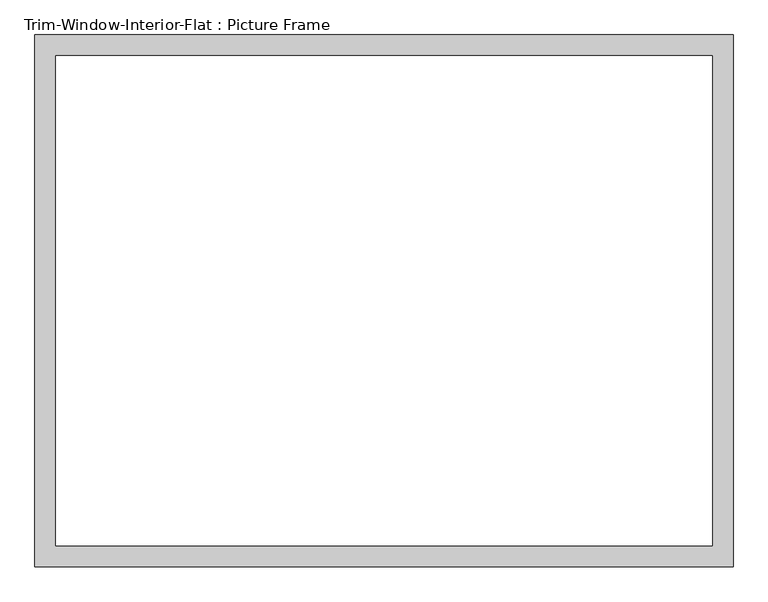
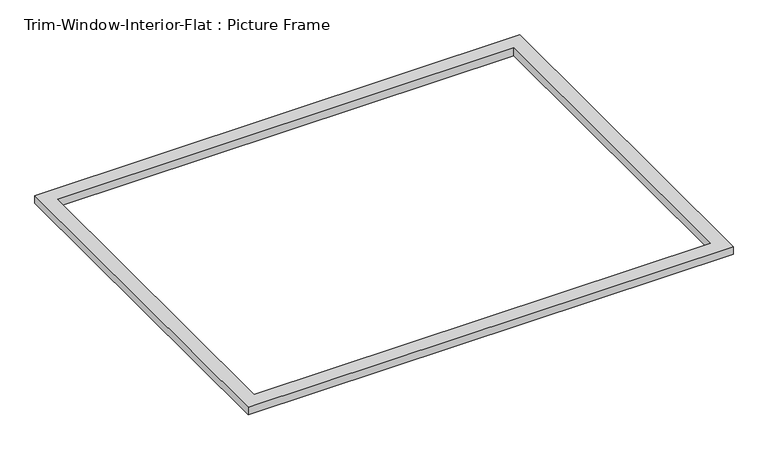
"""IFC4 building model written with IfcOpenShell, lengths in millimetres: proxy geometry, Trim-Window-Interior-Flat : Picture Frame."""

from ifc_helpers import new_model, si_unit, origin, origin_with_axes, place, context, project, spatial, polyline, outline, extrude, source, transform, mapped, element, save


def trim_window_interior_flat_picture_frame_f1d52788(model_context):
    return source(origin(), model_context, "Body", "SweptSolid", [
        extrude(outline(polyline([(958.85, 44.45), (958.85, -1416.05), (-958.85, -1416.05), (-958.85, 44.45), (958.85, 44.45)]), holes=[polyline([(901.7, -12.7), (-901.7, -12.7), (-901.7, -1358.9), (901.7, -1358.9), (901.7, -12.7)])]), origin_with_axes(), (0.0, 0.0, 1.0), 31.75),
    ])


if __name__ == "__main__":
    model = new_model("IFC4")
    model_context = context("Model", 3, world=origin())
    ifc_project = project(units=[si_unit("LENGTHUNIT", "METRE", prefix="MILLI")], contexts=[model_context])
    site = spatial("IfcSite", under=ifc_project)
    building = spatial("IfcBuilding", under=site)
    placement = place(None, origin())
    trim_window_interior_flat_picture_frame_shape = trim_window_interior_flat_picture_frame_f1d52788(model_context)
    element("IfcBuildingElementProxy", 1, Name="Trim-Window-Interior-Flat : Picture Frame", ObjectType="Trim-Window-Interior-Flat : Picture Frame", at=placement, inside=building, context=model_context, shape_type="MappedRepresentation", body=[
        mapped(trim_window_interior_flat_picture_frame_shape, transform((0.0, 0.0, 0.0), x_axis=(1.0, 0.0, 0.0), y_axis=(0.0, 1.0, 0.0), z_axis=(0.0, 0.0, 1.0))),
    ])
    save(model, "model.ifc")

# Revit data of these elements
# Type "Trim-Window-Interior-Flat : Picture Frame"
#   Trim Thickness_Picture Frame = 0' - 1 1/4"
#   Trim Width = 0' - 2 1/4"
#   Trim Thickness_with Sill = 0' - 0 3/4"
#   Sill Thickness = 0' - 1 1/4"
#   Opening Width [instance default] = 2' - 0"
#   Opening Height [instance default] = 3' - 0"
#   Default Elevation = 4' - 0"
#   Sill = no
#   Picture Frame = yes
#   Trim Material [instance default] = none
# Element 1 (IfcBuildingElementProxy, "Trim-Window-Interior-Flat : Picture Frame")
#   Opening Width = 6' - 0"
#   Opening Height = 4' - 6"
#   Trim Material = Wood - Stained
#   Materials on its faces: "Wood - Stained"
# Materials
#   "Wood - Stained": class "Wood", colour RGB 224 178 126, transparency 0, Cost = 0
